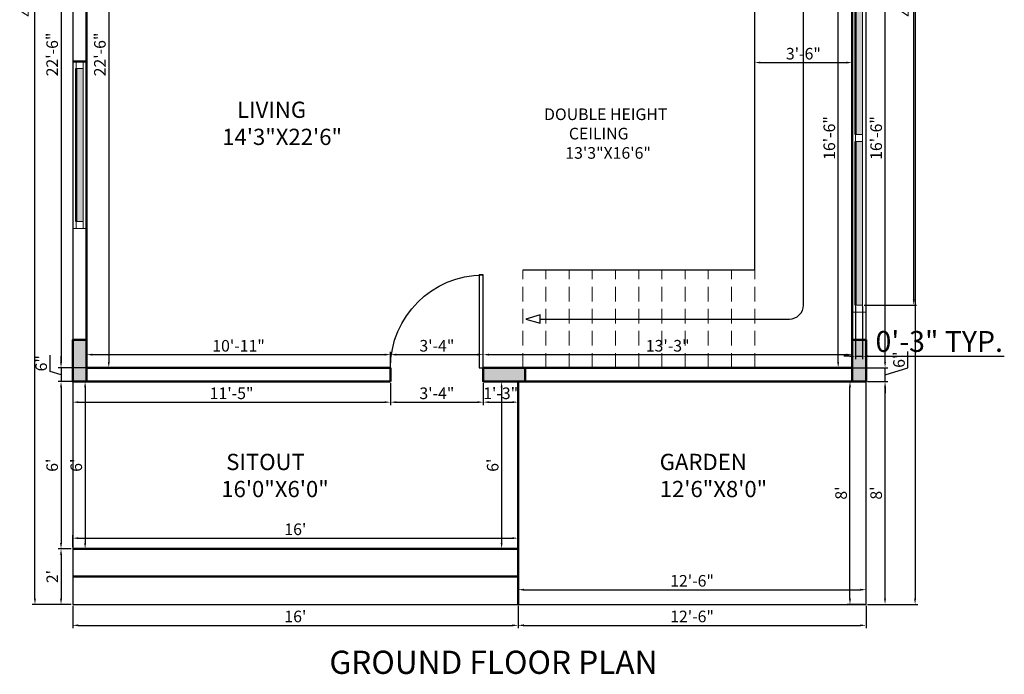
# Model space of a CAD drawing. Units: inches. Extents: x 3064 to 19385, y 846 to 15425.
# Tile 49 of 108: x 6020 to 6444, y 850 to 1132. Entities that reach past the tile are written whole.
import ezdxf

# ---------------------------------------------------------------- set-up
doc = ezdxf.new("R2010")
doc.units = ezdxf.units.IN
doc.linetypes.add('DASHED', pattern=[19.05, 12.7, -6.35])
for name, color, linetype, lineweight in [('A-ANNO-DIMS', 2, 'Continuous', 18), ('A-ANNO-TEXT', 7, 'Continuous', 25), ('A-AREA-IDEN', 3, 'Continuous', 18), ('A-COLS', 1, 'Continuous', 35), ('A-DOOR', 3, 'Continuous', 25), ('A-FLOR-STRS', 2, 'Continuous', 25), ('A-FLOR-STRS-OVHD', 2, 'DASHED', 18), ('A-GLAZ', 4, 'Continuous', 18), ('A-WALL', 7, 'Continuous', 50), ('C-PROP', 6, 'Continuous', 25)]:
    doc.layers.add(name, color=color, linetype=linetype, lineweight=lineweight)
doc.styles.get("Standard").update_dxf_attribs({"font": 'arial.ttf'})
doc.dimstyles.new('ISO-25', dxfattribs={"dimtxt": 9, "dimasz": 2.5, "dimexe": 1.25, "dimexo": 0.625, "dimtad": 1, "dimdec": 1, "dimlunit": 3, "dimtxsty": 'Standard', "dimcen": 2.5, "dimadec": 0, "dimazin": 0, "dimtfac": 1, "dimtdec": 1, "dimtmove": 0, "dimatfit": 3, "dimfxl": 1, "dimarcsym": 0})

# ---------------------------------------------------------------- blocks, each defined once
blk = doc.blocks.new('*U2')
for p, q in [((0, 0), (0, -6)), ((40, 0), (40, -6))]:
    blk.add_line(p, q)
blk.add_lwpolyline([(0, 0), (0, 40), (1.75, 40), (1.75, 0)], close=True)
blk.add_arc((0, 0), 40, 0, 90)
blk = doc.blocks.new('*D136')
at = {"layer": 'A-ANNO-DIMS', "color": 0, "lineweight": -2, "transparency": 16777216}
for p, q in [((6041.87, 1252.34), (6036.21, 1252.34)), ((6037.46, 1249.84), (6037.46, 984.84)), ((6047.87, 982.34), (6036.21, 982.34))]:
    blk.add_line(p, q, dxfattribs=at)
at = {"layer": 'A-ANNO-DIMS', "color": 0, "transparency": 16777216}
for points in [[(6037.05, 1249.84), (6037.88, 1249.84), (6037.46, 1252.34)], [(6037.05, 984.84), (6037.88, 984.84), (6037.46, 982.34)]]:
    blk.add_solid(points, dxfattribs=at)
at = {"layer": 'Defpoints', "color": 0, "transparency": 16777216}
for p in [(6042.49, 1252.34), (6037.46, 982.34), (6048.49, 982.34)]:
    blk.add_point(p, dxfattribs=at)
at = {"layer": 'A-ANNO-DIMS', "color": 0, "transparency": 16777216, "insert": (6034.29, 1117.34), "char_height": 5, "attachment_point": 5, "rotation": 90}
blk.add_mtext('22\'-6"', dxfattribs=at)
blk = doc.blocks.new('*D137')
at = {"layer": 'A-ANNO-DIMS', "color": 0, "lineweight": -2, "transparency": 16777216}
for p, q in [((6032.72, 980.76), (6032.72, 987.79)), ((6037.46, 984.84), (6037.46, 987.34)), ((6037.46, 979.34), (6032.72, 980.76)), ((6047.87, 982.34), (6036.21, 982.34)), ((6037.46, 982.34), (6037.46, 976.34)), ((6037.46, 982.34), (6037.46, 976.34)), ((6047.87, 976.34), (6036.21, 976.34)), ((6037.46, 973.84), (6037.46, 971.34))]:
    blk.add_line(p, q, dxfattribs=at)
at = {"layer": 'A-ANNO-DIMS', "color": 0, "transparency": 16777216}
for points in [[(6037.05, 984.84), (6037.88, 984.84), (6037.46, 982.34)], [(6037.05, 973.84), (6037.88, 973.84), (6037.46, 976.34)]]:
    blk.add_solid(points, dxfattribs=at)
at = {"layer": 'Defpoints', "color": 0, "transparency": 16777216}
for p in [(6048.49, 982.34), (6037.46, 976.34), (6048.49, 976.34)]:
    blk.add_point(p, dxfattribs=at)
at = {"layer": 'A-ANNO-DIMS', "color": 0, "transparency": 16777216, "insert": (6029.55, 984.27), "char_height": 5, "attachment_point": 5, "rotation": 90}
blk.add_mtext('6"', dxfattribs=at)
blk = doc.blocks.new('*D138')
at = {"layer": 'A-ANNO-DIMS', "color": 0, "lineweight": -2, "transparency": 16777216}
for p, q in [((6047.87, 976.34), (6036.21, 976.34)), ((6037.46, 973.84), (6037.46, 906.84)), ((6041.87, 904.34), (6036.21, 904.34))]:
    blk.add_line(p, q, dxfattribs=at)
at = {"layer": 'A-ANNO-DIMS', "color": 0, "transparency": 16777216}
for points in [[(6037.05, 973.84), (6037.88, 973.84), (6037.46, 976.34)], [(6037.05, 906.84), (6037.88, 906.84), (6037.46, 904.34)]]:
    blk.add_solid(points, dxfattribs=at)
at = {"layer": 'Defpoints', "color": 0, "transparency": 16777216}
for p in [(6048.49, 976.34), (6037.46, 904.34), (6042.49, 904.34)]:
    blk.add_point(p, dxfattribs=at)
at = {"layer": 'A-ANNO-DIMS', "color": 0, "transparency": 16777216, "insert": (6034.29, 940.34), "char_height": 5, "attachment_point": 5, "rotation": 90}
blk.add_mtext("6'", dxfattribs=at)
blk = doc.blocks.new('*D139')
at = {"layer": 'A-ANNO-DIMS', "color": 0, "lineweight": -2, "transparency": 16777216}
for p, q in [((6041.87, 904.34), (6036.21, 904.34)), ((6037.46, 901.84), (6037.46, 882.84)), ((6041.87, 880.34), (6036.21, 880.34))]:
    blk.add_line(p, q, dxfattribs=at)
at = {"layer": 'A-ANNO-DIMS', "color": 0, "transparency": 16777216}
for points in [[(6037.05, 901.84), (6037.88, 901.84), (6037.46, 904.34)], [(6037.05, 882.84), (6037.88, 882.84), (6037.46, 880.34)]]:
    blk.add_solid(points, dxfattribs=at)
at = {"layer": 'Defpoints', "color": 0, "transparency": 16777216}
for p in [(6042.49, 904.34), (6037.46, 880.34), (6042.49, 880.34)]:
    blk.add_point(p, dxfattribs=at)
at = {"layer": 'A-ANNO-DIMS', "color": 0, "transparency": 16777216, "insert": (6034.33, 892.34), "char_height": 5, "attachment_point": 5, "rotation": 90}
blk.add_mtext("2'", dxfattribs=at)
blk = doc.blocks.new('*D110')
at = {"layer": 'A-ANNO-DIMS', "color": 0, "lineweight": -2, "transparency": 16777216}
for p, q in [((6041.87, 1396.34), (6024.98, 1396.34)), ((6026.23, 882.84), (6026.23, 1393.84)), ((6041.87, 880.34), (6024.98, 880.34))]:
    blk.add_line(p, q, dxfattribs=at)
at = {"layer": 'A-ANNO-DIMS', "color": 0, "transparency": 16777216}
for points in [[(6025.81, 1393.84), (6026.64, 1393.84), (6026.23, 1396.34)], [(6025.81, 882.84), (6026.64, 882.84), (6026.23, 880.34)]]:
    blk.add_solid(points, dxfattribs=at)
at = {"layer": 'Defpoints', "color": 0, "transparency": 16777216}
for p in [(6026.23, 1396.34), (6042.49, 1396.34), (6042.49, 880.34)]:
    blk.add_point(p, dxfattribs=at)
at = {"layer": 'A-ANNO-DIMS', "color": 0, "transparency": 16777216, "insert": (6023.05, 1138.34), "char_height": 5, "attachment_point": 5, "rotation": 90}
blk.add_mtext("43'", dxfattribs=at)
blk = doc.blocks.new('*D111')
at = {"layer": 'A-ANNO-DIMS', "color": 0, "lineweight": -2, "transparency": 16777216}
for p, q in [((6042.49, 879.71), (6042.49, 870.08)), ((6234.49, 879.71), (6234.49, 870.08)), ((6044.99, 871.33), (6231.99, 871.33))]:
    blk.add_line(p, q, dxfattribs=at)
at = {"layer": 'A-ANNO-DIMS', "color": 0, "transparency": 16777216}
for points in [[(6044.99, 871.75), (6044.99, 870.91), (6042.49, 871.33)], [(6231.99, 871.75), (6231.99, 870.91), (6234.49, 871.33)]]:
    blk.add_solid(points, dxfattribs=at)
at = {"layer": 'Defpoints', "color": 0, "transparency": 16777216}
for p in [(6042.49, 880.34), (6234.49, 880.34), (6234.49, 871.33)]:
    blk.add_point(p, dxfattribs=at)
at = {"layer": 'A-ANNO-DIMS', "color": 0, "transparency": 16777216, "insert": (6138.49, 874.51), "char_height": 5, "attachment_point": 5}
blk.add_mtext("16'", dxfattribs=at)
blk = doc.blocks.new('*D112')
at = {"layer": 'A-ANNO-DIMS', "color": 0, "lineweight": -2, "transparency": 16777216}
for p, q in [((6234.49, 879.71), (6234.49, 870.08)), ((6384.49, 879.71), (6384.49, 870.08)), ((6236.99, 871.33), (6381.99, 871.33))]:
    blk.add_line(p, q, dxfattribs=at)
at = {"layer": 'A-ANNO-DIMS', "color": 0, "transparency": 16777216}
for points in [[(6236.99, 871.75), (6236.99, 870.91), (6234.49, 871.33)], [(6381.99, 871.75), (6381.99, 870.91), (6384.49, 871.33)]]:
    blk.add_solid(points, dxfattribs=at)
at = {"layer": 'Defpoints', "color": 0, "transparency": 16777216}
for p in [(6234.49, 880.34), (6384.49, 880.34), (6384.49, 871.33)]:
    blk.add_point(p, dxfattribs=at)
at = {"layer": 'A-ANNO-DIMS', "color": 0, "transparency": 16777216, "insert": (6309.49, 874.51), "char_height": 5, "attachment_point": 5}
blk.add_mtext('12\'-6"', dxfattribs=at)
blk = doc.blocks.new('*D113')
at = {"layer": 'A-ANNO-DIMS', "color": 0, "lineweight": -2, "transparency": 16777216}
for p, q in [((6385.12, 976.34), (6393.94, 976.34)), ((6392.69, 882.84), (6392.69, 973.84)), ((6385.12, 880.34), (6393.94, 880.34))]:
    blk.add_line(p, q, dxfattribs=at)
at = {"layer": 'A-ANNO-DIMS', "color": 0, "transparency": 16777216}
for points in [[(6392.27, 973.84), (6393.1, 973.84), (6392.69, 976.34)], [(6392.27, 882.84), (6393.1, 882.84), (6392.69, 880.34)]]:
    blk.add_solid(points, dxfattribs=at)
at = {"layer": 'Defpoints', "color": 0, "transparency": 16777216}
for p in [(6384.49, 976.34), (6392.69, 976.34), (6384.49, 880.34)]:
    blk.add_point(p, dxfattribs=at)
at = {"layer": 'A-ANNO-DIMS', "color": 0, "transparency": 16777216, "insert": (6389.51, 928.34), "char_height": 5, "attachment_point": 5, "rotation": 90}
blk.add_mtext("8'", dxfattribs=at)
blk = doc.blocks.new('*D114')
at = {"layer": 'A-ANNO-DIMS', "color": 0, "lineweight": -2, "transparency": 16777216}
for p, q in [((6402.53, 982.29), (6402.53, 989.32)), ((6392.69, 984.84), (6392.69, 987.34)), ((6379.12, 982.34), (6393.94, 982.34)), ((6392.69, 976.34), (6392.69, 982.34)), ((6392.69, 976.34), (6392.69, 982.34)), ((6392.69, 979.34), (6402.53, 982.29)), ((6385.12, 976.34), (6393.94, 976.34)), ((6392.69, 973.84), (6392.69, 971.34))]:
    blk.add_line(p, q, dxfattribs=at)
at = {"layer": 'A-ANNO-DIMS', "color": 0, "transparency": 16777216}
for points in [[(6392.27, 984.84), (6393.1, 984.84), (6392.69, 982.34)], [(6392.27, 973.84), (6393.1, 973.84), (6392.69, 976.34)]]:
    blk.add_solid(points, dxfattribs=at)
at = {"layer": 'Defpoints', "color": 0, "transparency": 16777216}
for p in [(6378.49, 982.34), (6392.69, 982.34), (6384.49, 976.34)]:
    blk.add_point(p, dxfattribs=at)
at = {"layer": 'A-ANNO-DIMS', "color": 0, "transparency": 16777216, "insert": (6399.35, 985.81), "char_height": 5, "attachment_point": 5, "rotation": 90}
blk.add_mtext('6"', dxfattribs=at)
blk = doc.blocks.new('*D106')
at = {"layer": 'A-ANNO-DIMS', "color": 0, "lineweight": -2, "transparency": 16777216}
for p, q in [((6379.12, 1180.34), (6393.94, 1180.34)), ((6392.69, 984.84), (6392.69, 1177.84)), ((6379.12, 982.34), (6393.94, 982.34))]:
    blk.add_line(p, q, dxfattribs=at)
at = {"layer": 'A-ANNO-DIMS', "color": 0, "transparency": 16777216}
for points in [[(6392.27, 1177.84), (6393.1, 1177.84), (6392.69, 1180.34)], [(6392.27, 984.84), (6393.1, 984.84), (6392.69, 982.34)]]:
    blk.add_solid(points, dxfattribs=at)
at = {"layer": 'Defpoints', "color": 0, "transparency": 16777216}
for p in [(6378.49, 1180.34), (6392.69, 1180.34), (6378.49, 982.34)]:
    blk.add_point(p, dxfattribs=at)
at = {"layer": 'A-ANNO-DIMS', "color": 0, "transparency": 16777216, "insert": (6389.51, 1081.34), "char_height": 5, "attachment_point": 5, "rotation": 90}
blk.add_mtext('16\'-6"', dxfattribs=at)
blk = doc.blocks.new('*D133')
at = {"layer": 'A-ANNO-DIMS', "color": 0, "lineweight": -2, "transparency": 16777216}
for p, q in [((6385.12, 1396.34), (6406.89, 1396.34)), ((6405.64, 1393.84), (6405.64, 882.84)), ((6385.12, 880.34), (6406.89, 880.34))]:
    blk.add_line(p, q, dxfattribs=at)
at = {"layer": 'A-ANNO-DIMS', "color": 0, "transparency": 16777216}
for points in [[(6405.22, 1393.84), (6406.05, 1393.84), (6405.64, 1396.34)], [(6405.22, 882.84), (6406.05, 882.84), (6405.64, 880.34)]]:
    blk.add_solid(points, dxfattribs=at)
at = {"layer": 'Defpoints', "color": 0, "transparency": 16777216}
for p in [(6384.49, 1396.34), (6384.49, 880.34), (6405.64, 880.34)]:
    blk.add_point(p, dxfattribs=at)
at = {"layer": 'A-ANNO-DIMS', "color": 0, "transparency": 16777216, "insert": (6402.46, 1138.34), "char_height": 5, "attachment_point": 5, "rotation": 90}
blk.add_mtext("43'", dxfattribs=at)
blk = doc.blocks.new('*D166')
at = {"layer": 'A-ANNO-DIMS', "color": 0, "lineweight": -2, "transparency": 16777216}
for p, q in [((6049.12, 1252.34), (6059.29, 1252.34)), ((6058.04, 1249.84), (6058.04, 984.84)), ((6049.12, 982.34), (6059.29, 982.34))]:
    blk.add_line(p, q, dxfattribs=at)
at = {"layer": 'A-ANNO-DIMS', "color": 0, "transparency": 16777216}
for points in [[(6057.63, 1249.84), (6058.46, 1249.84), (6058.04, 1252.34)], [(6057.63, 984.84), (6058.46, 984.84), (6058.04, 982.34)]]:
    blk.add_solid(points, dxfattribs=at)
at = {"layer": 'Defpoints', "color": 0, "transparency": 16777216}
for p in [(6048.49, 1252.34), (6048.49, 982.34), (6058.04, 982.34)]:
    blk.add_point(p, dxfattribs=at)
at = {"layer": 'A-ANNO-DIMS', "color": 0, "transparency": 16777216, "insert": (6054.87, 1117.34), "char_height": 5, "attachment_point": 5, "rotation": 90}
blk.add_mtext('22\'-6"', dxfattribs=at)
blk = doc.blocks.new('*D167')
at = {"layer": 'A-ANNO-DIMS', "color": 0, "lineweight": -2, "transparency": 16777216}
for p, q in [((6048.49, 982.96), (6048.49, 989.23)), ((6179.49, 982.96), (6179.49, 989.23)), ((6050.99, 987.98), (6176.99, 987.98))]:
    blk.add_line(p, q, dxfattribs=at)
at = {"layer": 'A-ANNO-DIMS', "color": 0, "transparency": 16777216}
for points in [[(6050.99, 988.4), (6050.99, 987.57), (6048.49, 987.98)], [(6176.99, 988.4), (6176.99, 987.57), (6179.49, 987.98)]]:
    blk.add_solid(points, dxfattribs=at)
at = {"layer": 'Defpoints', "color": 0, "transparency": 16777216}
for p in [(6179.49, 987.98), (6048.49, 982.34), (6179.49, 982.34)]:
    blk.add_point(p, dxfattribs=at)
at = {"layer": 'A-ANNO-DIMS', "color": 0, "transparency": 16777216, "insert": (6113.99, 991.16), "char_height": 5, "attachment_point": 5}
blk.add_mtext('10\'-11"', dxfattribs=at)
blk = doc.blocks.new('*D168')
at = {"layer": 'A-ANNO-DIMS', "color": 0, "lineweight": -2, "transparency": 16777216}
for p, q in [((6179.49, 982.96), (6179.49, 989.23)), ((6219.49, 982.96), (6219.49, 989.23)), ((6181.99, 987.98), (6216.99, 987.98))]:
    blk.add_line(p, q, dxfattribs=at)
at = {"layer": 'A-ANNO-DIMS', "color": 0, "transparency": 16777216}
for points in [[(6181.99, 988.4), (6181.99, 987.57), (6179.49, 987.98)], [(6216.99, 988.4), (6216.99, 987.57), (6219.49, 987.98)]]:
    blk.add_solid(points, dxfattribs=at)
at = {"layer": 'Defpoints', "color": 0, "transparency": 16777216}
for p in [(6219.49, 987.98), (6179.49, 982.34), (6219.49, 982.34)]:
    blk.add_point(p, dxfattribs=at)
at = {"layer": 'A-ANNO-DIMS', "color": 0, "transparency": 16777216, "insert": (6199.49, 991.16), "char_height": 5, "attachment_point": 5}
blk.add_mtext('3\'-4"', dxfattribs=at)
blk = doc.blocks.new('*D169')
at = {"layer": 'A-ANNO-DIMS', "color": 0, "lineweight": -2, "transparency": 16777216}
for p, q in [((6219.49, 982.96), (6219.49, 989.23)), ((6378.49, 982.96), (6378.49, 989.23)), ((6221.99, 987.98), (6375.99, 987.98))]:
    blk.add_line(p, q, dxfattribs=at)
at = {"layer": 'A-ANNO-DIMS', "color": 0, "transparency": 16777216}
for points in [[(6221.99, 988.4), (6221.99, 987.57), (6219.49, 987.98)], [(6375.99, 988.4), (6375.99, 987.57), (6378.49, 987.98)]]:
    blk.add_solid(points, dxfattribs=at)
at = {"layer": 'Defpoints', "color": 0, "transparency": 16777216}
for p in [(6378.49, 987.98), (6219.49, 982.34), (6378.49, 982.34)]:
    blk.add_point(p, dxfattribs=at)
at = {"layer": 'A-ANNO-DIMS', "color": 0, "transparency": 16777216, "insert": (6298.99, 991.16), "char_height": 5, "attachment_point": 5}
blk.add_mtext('13\'-3"', dxfattribs=at)
blk = doc.blocks.new('*D170')
at = {"layer": 'A-ANNO-DIMS', "color": 0, "lineweight": -2, "transparency": 16777216}
for p, q in [((6377.87, 1180.34), (6371.24, 1180.34)), ((6372.49, 984.84), (6372.49, 1177.84)), ((6377.87, 982.34), (6371.24, 982.34))]:
    blk.add_line(p, q, dxfattribs=at)
at = {"layer": 'A-ANNO-DIMS', "color": 0, "transparency": 16777216}
for points in [[(6372.07, 1177.84), (6372.9, 1177.84), (6372.49, 1180.34)], [(6372.07, 984.84), (6372.9, 984.84), (6372.49, 982.34)]]:
    blk.add_solid(points, dxfattribs=at)
at = {"layer": 'Defpoints', "color": 0, "transparency": 16777216}
for p in [(6372.49, 1180.34), (6378.49, 1180.34), (6378.49, 982.34)]:
    blk.add_point(p, dxfattribs=at)
at = {"layer": 'A-ANNO-DIMS', "color": 0, "transparency": 16777216, "insert": (6369.31, 1081.34), "char_height": 5, "attachment_point": 5, "rotation": 90}
blk.add_mtext('16\'-6"', dxfattribs=at)
blk = doc.blocks.new('*D173')
at = {"layer": 'A-ANNO-DIMS', "color": 0, "lineweight": -2, "transparency": 16777216}
for p, q in [((6043.12, 976.34), (6049.1, 976.34)), ((6047.85, 973.84), (6047.85, 906.84)), ((6043.12, 904.34), (6049.1, 904.34))]:
    blk.add_line(p, q, dxfattribs=at)
at = {"layer": 'A-ANNO-DIMS', "color": 0, "transparency": 16777216}
for points in [[(6047.44, 973.84), (6048.27, 973.84), (6047.85, 976.34)], [(6047.44, 906.84), (6048.27, 906.84), (6047.85, 904.34)]]:
    blk.add_solid(points, dxfattribs=at)
at = {"layer": 'Defpoints', "color": 0, "transparency": 16777216}
for p in [(6042.49, 976.34), (6042.49, 904.34), (6047.85, 904.34)]:
    blk.add_point(p, dxfattribs=at)
at = {"layer": 'A-ANNO-DIMS', "color": 0, "transparency": 16777216, "insert": (6044.68, 940.34), "char_height": 5, "attachment_point": 5, "rotation": 90}
blk.add_mtext("6'", dxfattribs=at)
blk = doc.blocks.new('*D174')
at = {"layer": 'A-ANNO-DIMS', "color": 0, "lineweight": -2, "transparency": 16777216}
for p, q in [((6042.49, 975.71), (6042.49, 966.25)), ((6179.49, 975.71), (6179.49, 966.25)), ((6044.99, 967.5), (6176.99, 967.5))]:
    blk.add_line(p, q, dxfattribs=at)
at = {"layer": 'A-ANNO-DIMS', "color": 0, "transparency": 16777216}
for points in [[(6044.99, 967.92), (6044.99, 967.09), (6042.49, 967.5)], [(6176.99, 967.92), (6176.99, 967.09), (6179.49, 967.5)]]:
    blk.add_solid(points, dxfattribs=at)
at = {"layer": 'Defpoints', "color": 0, "transparency": 16777216}
for p in [(6042.49, 976.34), (6179.49, 976.34), (6179.49, 967.5)]:
    blk.add_point(p, dxfattribs=at)
at = {"layer": 'A-ANNO-DIMS', "color": 0, "transparency": 16777216, "insert": (6110.99, 970.68), "char_height": 5, "attachment_point": 5}
blk.add_mtext('11\'-5"', dxfattribs=at)
blk = doc.blocks.new('*D175')
at = {"layer": 'A-ANNO-DIMS', "color": 0, "lineweight": -2, "transparency": 16777216}
for p, q in [((6179.49, 975.71), (6179.49, 966.25)), ((6219.49, 975.71), (6219.49, 966.25)), ((6181.99, 967.5), (6216.99, 967.5))]:
    blk.add_line(p, q, dxfattribs=at)
at = {"layer": 'A-ANNO-DIMS', "color": 0, "transparency": 16777216}
for points in [[(6181.99, 967.92), (6181.99, 967.09), (6179.49, 967.5)], [(6216.99, 967.92), (6216.99, 967.09), (6219.49, 967.5)]]:
    blk.add_solid(points, dxfattribs=at)
at = {"layer": 'Defpoints', "color": 0, "transparency": 16777216}
for p in [(6179.49, 976.34), (6219.49, 976.34), (6219.49, 967.5)]:
    blk.add_point(p, dxfattribs=at)
at = {"layer": 'A-ANNO-DIMS', "color": 0, "transparency": 16777216, "insert": (6199.49, 970.68), "char_height": 5, "attachment_point": 5}
blk.add_mtext('3\'-4"', dxfattribs=at)
blk = doc.blocks.new('*D176')
at = {"layer": 'A-ANNO-DIMS', "color": 0, "lineweight": -2, "transparency": 16777216}
for p, q in [((6219.49, 975.71), (6219.49, 966.25)), ((6234.49, 975.71), (6234.49, 966.25)), ((6221.99, 967.5), (6231.99, 967.5))]:
    blk.add_line(p, q, dxfattribs=at)
at = {"layer": 'A-ANNO-DIMS', "color": 0, "transparency": 16777216}
for points in [[(6221.99, 967.92), (6221.99, 967.09), (6219.49, 967.5)], [(6231.99, 967.92), (6231.99, 967.09), (6234.49, 967.5)]]:
    blk.add_solid(points, dxfattribs=at)
at = {"layer": 'Defpoints', "color": 0, "transparency": 16777216}
for p in [(6219.49, 976.34), (6234.49, 976.34), (6234.49, 967.5)]:
    blk.add_point(p, dxfattribs=at)
at = {"layer": 'A-ANNO-DIMS', "color": 0, "transparency": 16777216, "insert": (6226.99, 970.68), "char_height": 5, "attachment_point": 5}
blk.add_mtext('1\'-3"', dxfattribs=at)
blk = doc.blocks.new('*D177')
at = {"layer": 'A-ANNO-DIMS', "color": 0, "lineweight": -2, "transparency": 16777216}
for p, q in [((6042.49, 904.96), (6042.49, 910.15)), ((6044.99, 908.9), (6231.99, 908.9)), ((6234.49, 904.96), (6234.49, 910.15))]:
    blk.add_line(p, q, dxfattribs=at)
at = {"layer": 'A-ANNO-DIMS', "color": 0, "transparency": 16777216}
for points in [[(6044.99, 909.32), (6044.99, 908.49), (6042.49, 908.9)], [(6231.99, 909.32), (6231.99, 908.49), (6234.49, 908.9)]]:
    blk.add_solid(points, dxfattribs=at)
at = {"layer": 'Defpoints', "color": 0, "transparency": 16777216}
for p in [(6234.49, 908.9), (6042.49, 904.34), (6234.49, 904.34)]:
    blk.add_point(p, dxfattribs=at)
at = {"layer": 'A-ANNO-DIMS', "color": 0, "transparency": 16777216, "insert": (6138.49, 912.08), "char_height": 5, "attachment_point": 5}
blk.add_mtext("16'", dxfattribs=at)
blk = doc.blocks.new('*D178')
at = {"layer": 'A-ANNO-DIMS', "color": 0, "lineweight": -2, "transparency": 16777216}
for p, q in [((6233.87, 976.34), (6226.14, 976.34)), ((6227.39, 973.84), (6227.39, 906.84)), ((6233.87, 904.34), (6226.14, 904.34))]:
    blk.add_line(p, q, dxfattribs=at)
at = {"layer": 'A-ANNO-DIMS', "color": 0, "transparency": 16777216}
for points in [[(6226.97, 973.84), (6227.81, 973.84), (6227.39, 976.34)], [(6226.97, 906.84), (6227.81, 906.84), (6227.39, 904.34)]]:
    blk.add_solid(points, dxfattribs=at)
at = {"layer": 'Defpoints', "color": 0, "transparency": 16777216}
for p in [(6234.49, 976.34), (6227.39, 904.34), (6234.49, 904.34)]:
    blk.add_point(p, dxfattribs=at)
at = {"layer": 'A-ANNO-DIMS', "color": 0, "transparency": 16777216, "insert": (6224.21, 940.34), "char_height": 5, "attachment_point": 5, "rotation": 90}
blk.add_mtext("6'", dxfattribs=at)
blk = doc.blocks.new('*D179')
at = {"layer": 'A-ANNO-DIMS', "color": 0, "lineweight": -2, "transparency": 16777216}
for p, q in [((6234.49, 880.96), (6234.49, 887.94)), ((6384.49, 880.96), (6384.49, 887.94)), ((6236.99, 886.69), (6381.99, 886.69))]:
    blk.add_line(p, q, dxfattribs=at)
at = {"layer": 'A-ANNO-DIMS', "color": 0, "transparency": 16777216}
for points in [[(6236.99, 887.11), (6236.99, 886.28), (6234.49, 886.69)], [(6381.99, 887.11), (6381.99, 886.28), (6384.49, 886.69)]]:
    blk.add_solid(points, dxfattribs=at)
at = {"layer": 'Defpoints', "color": 0, "transparency": 16777216}
for p in [(6384.49, 886.69), (6234.49, 880.34), (6384.49, 880.34)]:
    blk.add_point(p, dxfattribs=at)
at = {"layer": 'A-ANNO-DIMS', "color": 0, "transparency": 16777216, "insert": (6309.49, 889.87), "char_height": 5, "attachment_point": 5}
blk.add_mtext('12\'-6"', dxfattribs=at)
blk = doc.blocks.new('*D180')
at = {"layer": 'A-ANNO-DIMS', "color": 0, "lineweight": -2, "transparency": 16777216}
for p, q in [((6383.87, 976.34), (6376.32, 976.34)), ((6377.57, 882.84), (6377.57, 973.84)), ((6383.87, 880.34), (6376.32, 880.34))]:
    blk.add_line(p, q, dxfattribs=at)
at = {"layer": 'A-ANNO-DIMS', "color": 0, "transparency": 16777216}
for points in [[(6377.15, 973.84), (6377.99, 973.84), (6377.57, 976.34)], [(6377.15, 882.84), (6377.99, 882.84), (6377.57, 880.34)]]:
    blk.add_solid(points, dxfattribs=at)
at = {"layer": 'Defpoints', "color": 0, "transparency": 16777216}
for p in [(6377.57, 976.34), (6384.49, 976.34), (6384.49, 880.34)]:
    blk.add_point(p, dxfattribs=at)
at = {"layer": 'A-ANNO-DIMS', "color": 0, "transparency": 16777216, "insert": (6374.39, 928.34), "char_height": 5, "attachment_point": 5, "rotation": 90}
blk.add_mtext("8'", dxfattribs=at)
blk = doc.blocks.new('*D186')
at = {"layer": 'A-ANNO-DIMS', "color": 0, "lineweight": -2, "transparency": 16777216}
for p, q in [((6336.49, 1114.47), (6336.49, 1115.09)), ((6338.99, 1113.84), (6375.99, 1113.84)), ((6378.49, 1114.47), (6378.49, 1115.09))]:
    blk.add_line(p, q, dxfattribs=at)
at = {"layer": 'A-ANNO-DIMS', "color": 0, "transparency": 16777216}
for points in [[(6338.99, 1114.26), (6338.99, 1113.43), (6336.49, 1113.84)], [(6375.99, 1114.26), (6375.99, 1113.43), (6378.49, 1113.84)]]:
    blk.add_solid(points, dxfattribs=at)
at = {"layer": 'Defpoints', "color": 0, "transparency": 16777216}
for p in [(6336.49, 1113.84), (6378.49, 1113.84), (6378.49, 1113.84)]:
    blk.add_point(p, dxfattribs=at)
at = {"layer": 'A-ANNO-DIMS', "color": 0, "transparency": 16777216, "insert": (6357.49, 1117.02), "char_height": 5, "attachment_point": 5}
blk.add_mtext('3\'-6"', dxfattribs=at)
blk = doc.blocks.new('WIN-1800-PAIR')
h = blk.add_hatch(color=256)
h.dxf.hatch_style = 1
h.paths.add_polyline_path([(0, 0), (3, 0), (3, 70.5), (0, 70.5)])
h.paths.add_polyline_path([(3, 144), (0, 144), (0, 73.5), (3, 73.5)])
blk.add_line((3, 144), (3, 73.5))
blk.add_lwpolyline([(3, 144), (0, 144), (0, 147), (3, 147)], close=True)
blk = doc.blocks.new('WIN-2000')
blk.add_line((3, 0), (3, 70.5))
blk.add_lwpolyline([(3, 70.5), (0, 70.5), (0, 73.5), (3, 73.5)], close=True)
blk = doc.blocks.new('WIN-1900')
blk.add_line((3, 0), (3, 66))
blk.add_lwpolyline([(3, 66), (0, 66), (0, 69), (3, 69)], close=True)
blk = doc.blocks.new('*D445')
at = {"layer": 'A-ANNO-DIMS', "color": 0, "lineweight": -2, "transparency": 16777216}
for p, q in [((6405.04, 1156.34), (6405.04, 1357.14)), ((6383.62, 1156.34), (6406.29, 1156.34)), ((6405.04, 1011.84), (6405.04, 1153.84)), ((6383.62, 1009.34), (6406.29, 1009.34))]:
    blk.add_line(p, q, dxfattribs=at)
at = {"layer": 'A-ANNO-DIMS', "color": 0, "transparency": 16777216}
for points in [[(6404.63, 1153.84), (6405.46, 1153.84), (6405.04, 1156.34)], [(6404.63, 1011.84), (6405.46, 1011.84), (6405.04, 1009.34)]]:
    blk.add_solid(points, dxfattribs=at)
at = {"layer": 'Defpoints', "color": 0, "transparency": 16777216}
for p in [(6382.99, 1156.34), (6405.04, 1156.34), (6382.99, 1009.34)]:
    blk.add_point(p, dxfattribs=at)
at = {"layer": 'A-ANNO-DIMS', "color": 0, "transparency": 16777216, "insert": (6399.76, 1257.99), "char_height": 9, "attachment_point": 5, "rotation": 90}
blk.add_mtext('WINDOW W1800 PAIR 12\'-3" TYP.', dxfattribs=at)
blk = doc.blocks.new('*D446')
at = {"layer": 'A-ANNO-DIMS', "color": 0, "lineweight": -2, "transparency": 16777216}
for p, q in [((6379.99, 1008.71), (6379.99, 986.04)), ((6382.99, 1008.71), (6382.99, 986.04)), ((6377.49, 987.29), (6374.99, 987.29)), ((6379.99, 987.29), (6382.99, 987.29)), ((6385.49, 987.29), (6444.1, 987.29))]:
    blk.add_line(p, q, dxfattribs=at)
at = {"layer": 'A-ANNO-DIMS', "color": 0, "transparency": 16777216}
for points in [[(6377.49, 987.71), (6377.49, 986.87), (6379.99, 987.29)], [(6385.49, 987.71), (6385.49, 986.87), (6382.99, 987.29)]]:
    blk.add_solid(points, dxfattribs=at)
at = {"layer": 'Defpoints', "color": 0, "transparency": 16777216}
for p in [(6379.99, 1009.34), (6382.99, 1009.34), (6382.99, 987.29)]:
    blk.add_point(p, dxfattribs=at)
at = {"layer": 'A-ANNO-DIMS', "color": 0, "transparency": 16777216, "insert": (6416.05, 992.51), "char_height": 9, "attachment_point": 5}
blk.add_mtext('0\'-3" TYP.', dxfattribs=at)

msp = doc.modelspace()

# ---------------------------------------------------------------- hatches: boundary and pattern name
at = {"layer": 'A-COLS'}
h = msp.add_hatch(color=256, dxfattribs=at)
h.dxf.hatch_style = 1
h.paths.add_polyline_path([(6042.49, 976.34), (6048.49, 976.34), (6048.49, 994.34), (6042.49, 994.34)])
h = msp.add_hatch(color=256, dxfattribs=at)
h.dxf.hatch_style = 1
h.paths.add_polyline_path([(6378.49, 976.34), (6384.49, 976.34), (6384.49, 994.34), (6378.49, 994.34)])
h = msp.add_hatch(color=256, dxfattribs=at)
h.dxf.hatch_style = 1
h.paths.add_polyline_path([(6237.49, 976.34), (6237.49, 982.34), (6219.49, 982.34), (6219.49, 976.34)])
at = {"layer": 'A-GLAZ'}
h = msp.add_hatch(color=256, dxfattribs=at)
h.dxf.hatch_style = 1
h.paths.add_polyline_path([(6043.99, 1045.34), (6046.99, 1045.34), (6046.99, 1111.34), (6043.99, 1111.34)])

# ---------------------------------------------------------------- linework, layer by layer
at = {"layer": 'A-FLOR-STRS'}
for q in [(6336.49, 1180.34), (6236.49, 1024.34)]:
    msp.add_line((6336.49, 1024.34), q, dxfattribs=at)
msp.add_lwpolyline([(6243.98, 1003.34), (6351.49, 1003.34, 0.414214), (6357.49, 1009.34), (6357.49, 1153.34, 0.414214), (6351.49, 1159.34), (6224.49, 1159.34)], format="xyb", dxfattribs=at)
msp.add_lwpolyline([(6237.79, 1003.34), (6243.98, 1001.61), (6243.98, 1005.07)], close=True, dxfattribs=at)
at = {"layer": 'A-FLOR-STRS-OVHD', "ltscale": 0.5}
for p, q in [((6236.49, 982.34), (6236.49, 1024.34)), ((6246.49, 982.34), (6246.49, 1024.34)), ((6256.49, 982.34), (6256.49, 1024.34)), ((6266.49, 982.34), (6266.49, 1024.34)), ((6276.49, 982.34), (6276.49, 1024.34)), ((6286.49, 982.34), (6286.49, 1024.34)), ((6296.49, 982.34), (6296.49, 1024.34)), ((6306.49, 982.34), (6306.49, 1024.34)), ((6316.49, 982.34), (6316.49, 1024.34)), ((6326.49, 982.34), (6326.49, 1024.34)), ((6336.49, 982.34), (6336.49, 1024.34))]:
    msp.add_line(p, q, dxfattribs=at)
at = {"layer": 'A-GLAZ'}
for p, q in [((6048.49, 1042.34), (6042.49, 1042.34)), ((6384.49, 1006.34), (6378.49, 1006.34)), ((6384.49, 1006.34), (6378.49, 1006.34))]:
    msp.add_line(p, q, dxfattribs=at)
for points in [[(6046.99, 1042.34), (6043.99, 1042.34), (6043.99, 1045.34), (6046.99, 1045.34)], [(6382.99, 1006.34), (6379.99, 1006.34), (6379.99, 1009.34), (6382.99, 1009.34)]]:
    msp.add_lwpolyline(points, close=True, dxfattribs=at)
at = {"layer": 'A-WALL'}
for p, q in [((6048.49, 1390.34), (6048.49, 982.34)), ((6378.49, 982.34), (6378.49, 1180.34)), ((6379.99, 1153.34), (6379.99, 1082.84)), ((6048.49, 1114.34), (6042.49, 1114.34)), ((6043.99, 1045.34), (6043.99, 1111.34)), ((6379.99, 1009.34), (6379.99, 1079.84)), ((6179.49, 982.34), (6048.49, 982.34)), ((6179.49, 976.34), (6179.49, 982.34)), ((6378.49, 982.34), (6219.49, 982.34)), ((6219.49, 976.34), (6219.49, 982.34)), ((6179.49, 976.34), (6042.49, 976.34)), ((6384.49, 976.34), (6219.49, 976.34)), ((6234.49, 976.34), (6234.49, 880.34)), ((6042.49, 904.34), (6234.49, 904.34)), ((6042.49, 892.34), (6234.49, 892.34))]:
    msp.add_line(p, q, dxfattribs=at)
for points in [[(6048.49, 976.34), (6048.49, 994.34), (6042.49, 994.34), (6042.49, 976.34)], [(6384.49, 976.34), (6384.49, 994.34), (6378.49, 994.34), (6378.49, 976.34)], [(6237.49, 982.34), (6219.49, 982.34), (6219.49, 976.34), (6237.49, 976.34)]]:
    msp.add_lwpolyline(points, close=True, dxfattribs=at)
at = {"layer": 'C-PROP'}
for p, q in [((6042.49, 1396.34), (6042.49, 880.34)), ((6384.49, 880.34), (6384.49, 1396.34)), ((6042.49, 880.34), (6384.49, 880.34))]:
    msp.add_line(p, q, dxfattribs=at)

# ---------------------------------------------------------------- block references
at = {"layer": 'A-DOOR', "xscale": -1}
msp.add_blockref('*U2', (6219.49, 982.34), dxfattribs=at)
at = {"layer": 'A-GLAZ'}
for name, p in [('WIN-1800-PAIR', (6379.99, 1009.34)), ('WIN-1900', (6043.99, 1045.34)), ('WIN-2000', (6379.99, 1009.34))]:
    msp.add_blockref(name, p, dxfattribs=at)

# ---------------------------------------------------------------- texts
at = {"layer": 'A-ANNO-TEXT', "insert": (6153.16, 860.41), "char_height": 10, "attachment_point": 1}
msp.add_mtext_dynamic_manual_height_columns('GROUND FLOOR PLAN', width=200.9739, gutter_width=12.5, heights=[0], dxfattribs=at)
at = {"layer": 'A-AREA-IDEN', "attachment_point": 1}
for s, width, insert, char_height in [('   LIVING\\P14\'3"X22\'6"', 67.5924, (6106.95, 1097), 7), ('DOUBLE HEIGHT \\P       CEILING            \\P      13\'3"X16\'6"', 57.0817, (6245.7, 1094.07), 5), (' SITOUT\\P16\'0"X6\'0"', 67.5924, (6106.53, 945.24), 7), ('GARDEN\\P12\'6"X8\'0"', 67.5924, (6295.54, 945.24), 7)]:
    msp.add_mtext_dynamic_manual_height_columns(s, width=width, gutter_width=12.5, heights=[0], dxfattribs=dict(at, insert=insert, char_height=char_height))

# ---------------------------------------------------------------- dimensions: what is measured, and where the dimension line sits
at = {"layer": 'A-ANNO-DIMS'}
for base, p1, p2, override, picture, middle in [((6026.23, 1396.34), (6042.49, 880.34), (6042.49, 1396.34), {"dimtxt": 5, "dimclrd": 0, "dimclre": 0, "dimclrt": 0}, '*D110', (6023.05, 1138.34)), ((6405.64, 880.34), (6384.49, 1396.34), (6384.49, 880.34), {"dimtxt": 5, "dimclrd": 0, "dimclre": 0, "dimclrt": 0}, '*D133', (6402.46, 1138.34)), ((6037.46, 982.34), (6042.49, 1252.34), (6048.49, 982.34), {"dimtxt": 5, "dimclrd": 0, "dimclre": 0, "dimclrt": 0, "dimtmove": 1}, '*D136', (6034.29, 1117.34)), ((6058.04, 982.34), (6048.49, 1252.34), (6048.49, 982.34), {"dimtxt": 5, "dimclrd": 0, "dimclre": 0, "dimclrt": 0}, '*D166', (6054.87, 1117.34)), ((6372.49, 1180.34), (6378.49, 982.34), (6378.49, 1180.34), {"dimtxt": 5, "dimclrd": 0, "dimclre": 0, "dimclrt": 0}, '*D170', (6369.31, 1081.34)), ((6392.69, 1180.34), (6378.49, 982.34), (6378.49, 1180.34), {"dimtxt": 5, "dimclrd": 0, "dimclre": 0, "dimclrt": 0, "dimtmove": 1}, '*D106', (6389.51, 1081.34)), ((6392.69, 982.34), (6384.49, 976.34), (6378.49, 982.34), {"dimtxt": 5, "dimclrd": 0, "dimclre": 0, "dimclrt": 0, "dimtmove": 1}, '*D114', (6399.35, 982.92)), ((6037.46, 976.34), (6048.49, 982.34), (6048.49, 976.34), {"dimtxt": 5, "dimclrd": 0, "dimclre": 0, "dimclrt": 0, "dimtmove": 1}, '*D137', (6029.55, 981.39)), ((6037.46, 904.34), (6048.49, 976.34), (6042.49, 904.34), {"dimtxt": 5, "dimclrd": 0, "dimclre": 0, "dimclrt": 0, "dimtmove": 1}, '*D138', (6034.29, 940.34)), ((6047.85, 904.34), (6042.49, 976.34), (6042.49, 904.34), {"dimtxt": 5, "dimclrd": 0, "dimclre": 0, "dimclrt": 0}, '*D173', (6044.68, 940.34)), ((6227.39, 904.34), (6234.49, 976.34), (6234.49, 904.34), {"dimtxt": 5, "dimclrd": 0, "dimclre": 0, "dimclrt": 0}, '*D178', (6224.21, 940.34)), ((6377.57, 976.34), (6384.49, 880.34), (6384.49, 976.34), {"dimtxt": 5, "dimclrd": 0, "dimclre": 0, "dimclrt": 0}, '*D180', (6374.39, 928.34)), ((6392.69, 976.34), (6384.49, 880.34), (6384.49, 976.34), {"dimtxt": 5, "dimclrd": 0, "dimclre": 0, "dimclrt": 0}, '*D113', (6389.51, 928.34)), ((6037.46, 880.34), (6042.49, 904.34), (6042.49, 880.34), {"dimtxt": 5, "dimclrd": 0, "dimclre": 0, "dimclrt": 0, "dimtmove": 1}, '*D139', (6034.33, 892.34))]:
    dim = msp.add_linear_dim(base=base, p1=p1, p2=p2, angle=90, dimstyle='ISO-25', override=override, dxfattribs=at)
    dim.commit()
    dim.dimension.update_dxf_attribs({"geometry": picture, "text_midpoint": middle})
dim = msp.add_linear_dim(base=(6405.04, 1156.34), p1=(6382.99, 1009.34), p2=(6382.99, 1156.34), angle=90, text='WINDOW W1800 PAIR <> TYP.', dimstyle='ISO-25', override={"dimdec": 1, "dimrnd": 0, "dimzin": 1, "dimlunit": 4, "dimfrac": 2}, dxfattribs=at)
dim.commit()
dim.dimension.update_dxf_attribs({"geometry": '*D445', "text_midpoint": (6399.76, 1257.99)})
for base, p1, p2, override, picture, middle in [((6378.49, 1113.84), (6336.49, 1113.84), (6378.49, 1113.84), {"dimtxt": 5, "dimclrd": 0, "dimclre": 0, "dimclrt": 0}, '*D186', (6357.49, 1117.02)), ((6179.49, 987.98), (6048.49, 982.34), (6179.49, 982.34), {"dimtxt": 5, "dimclrd": 0, "dimclre": 0, "dimclrt": 0}, '*D167', (6113.99, 991.16)), ((6219.49, 987.98), (6179.49, 982.34), (6219.49, 982.34), {"dimtxt": 5, "dimclrd": 0, "dimclre": 0, "dimclrt": 0, "dimtmove": 1}, '*D168', (6199.49, 991.16)), ((6378.49, 987.98), (6219.49, 982.34), (6378.49, 982.34), {"dimtxt": 5, "dimclrd": 0, "dimclre": 0, "dimclrt": 0, "dimtmove": 1}, '*D169', (6298.99, 991.16)), ((6179.49, 967.5), (6042.49, 976.34), (6179.49, 976.34), {"dimtxt": 5, "dimclrd": 0, "dimclre": 0, "dimclrt": 0}, '*D174', (6110.99, 970.68)), ((6219.49, 967.5), (6179.49, 976.34), (6219.49, 976.34), {"dimtxt": 5, "dimclrd": 0, "dimclre": 0, "dimclrt": 0, "dimtmove": 1}, '*D175', (6199.49, 970.68)), ((6234.49, 967.5), (6219.49, 976.34), (6234.49, 976.34), {"dimtxt": 5, "dimclrd": 0, "dimclre": 0, "dimclrt": 0, "dimtmove": 1}, '*D176', (6226.99, 970.68)), ((6234.49, 908.9), (6042.49, 904.34), (6234.49, 904.34), {"dimtxt": 5, "dimclrd": 0, "dimclre": 0, "dimclrt": 0}, '*D177', (6138.49, 912.08)), ((6384.49, 886.69), (6234.49, 880.34), (6384.49, 880.34), {"dimtxt": 5, "dimclrd": 0, "dimclre": 0, "dimclrt": 0}, '*D179', (6309.49, 889.87)), ((6234.49, 871.33), (6042.49, 880.34), (6234.49, 880.34), {"dimtxt": 5, "dimclrd": 0, "dimclre": 0, "dimclrt": 0}, '*D111', (6138.49, 874.51)), ((6384.49, 871.33), (6234.49, 880.34), (6384.49, 880.34), {"dimtxt": 5, "dimclrd": 0, "dimclre": 0, "dimclrt": 0, "dimtmove": 1}, '*D112', (6309.49, 874.51))]:
    dim = msp.add_linear_dim(base=base, p1=p1, p2=p2, dimstyle='ISO-25', override=override, dxfattribs=at)
    dim.commit()
    dim.dimension.update_dxf_attribs({"geometry": picture, "text_midpoint": middle})
dim = msp.add_linear_dim(base=(6382.99, 987.29), p1=(6379.99, 1009.34), p2=(6382.99, 1009.34), text='<> TYP.', dimstyle='ISO-25', override={"dimdec": 1, "dimrnd": 0, "dimzin": 1, "dimlunit": 4, "dimfrac": 2}, dxfattribs=at)
dim.commit()
dim.dimension.update_dxf_attribs({"geometry": '*D446', "text_midpoint": (6416.05, 992.51)})

doc.saveas('drawing.dxf')
